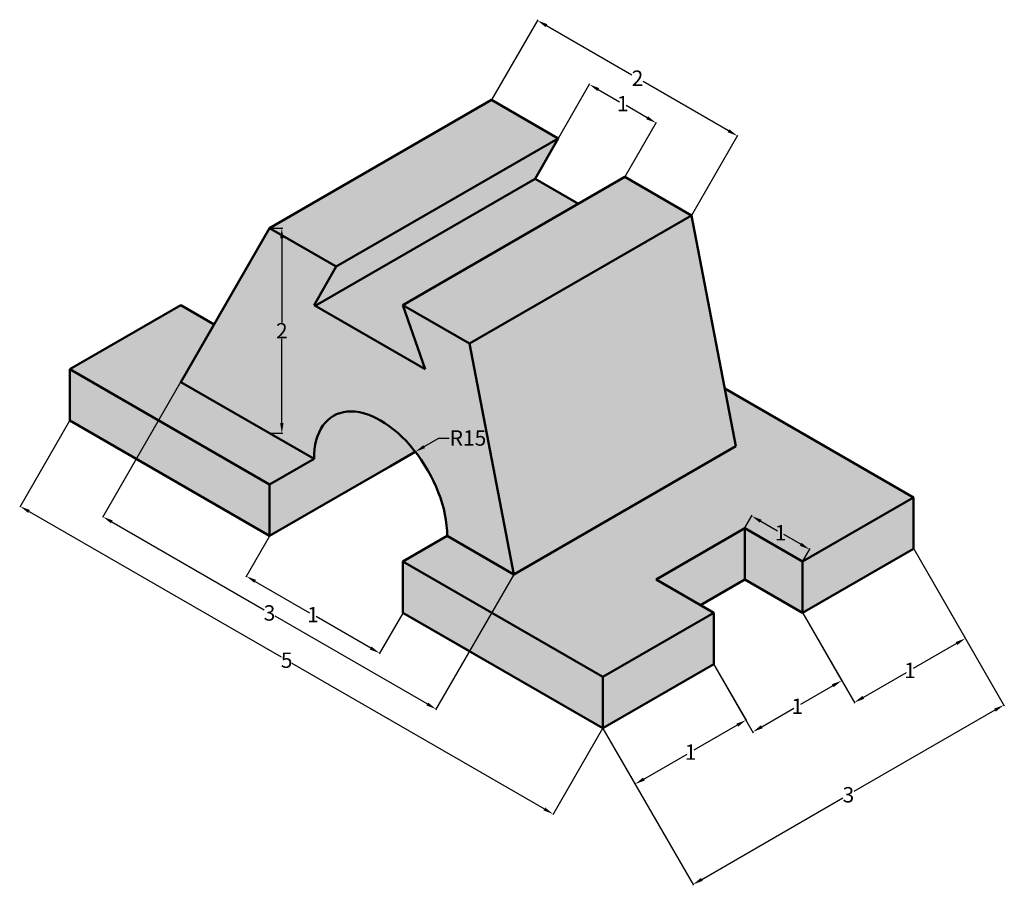
# Model space of a CAD drawing. Units: inches. Extents: x 162 to 354, y 120 to 289.
import ezdxf
from ezdxf import colors
from ezdxf.entities.mleader import LeaderData, LeaderLine
from ezdxf.math import Vec2, Vec3

# ---------------------------------------------------------------- set-up
doc = ezdxf.new("R2010")
doc.units = ezdxf.units.IN
doc.header["$MEASUREMENT"] = 0
for name, color, linetype, lineweight in [('M-DIMS', 2, 'Continuous', 25), ('M-HATC', 252, 'Continuous', 18), ('M-OUTL', 7, 'Continuous', 50), ('M-TEXT', 7, 'Continuous', 25)]:
    doc.layers.add(name, color=color, linetype=linetype, lineweight=lineweight)
doc.styles.get("Standard").update_dxf_attribs({"font": 'arial.ttf'})
doc.dimstyles.get("Standard").update_dxf_attribs({"dimtxt": 3, "dimasz": 2, "dimexe": 0.18, "dimexo": 0.0625, "dimgap": 0.09, "dimtad": 0, "dimtih": 1, "dimtoh": 1, "dimdec": 0, "dimzin": 0, "dimdsep": 46, "dimtxsty": 'Standard', "dimcen": 0.09, "dimadec": 0, "dimazin": 0, "dimtfac": 1, "dimtdec": 0, "dimtofl": 0, "dimtmove": 0, "dimatfit": 3, "dimfxl": 1, "dimtolj": 1, "dimtzin": 0, "dimarcsym": 0})

# ---------------------------------------------------------------- blocks, each defined once
blk = doc.blocks.new('*D23')
at = {"layer": 'Defpoints', "color": 0, "transparency": 16777216}
for p in [(172.0397916164236, 210.9806443557733), (275.9628400705561, 150.9806443557734), (266.299650434846, 134.2435089435503)]:
    blk.add_point(p, dxfattribs=at)
at = {"layer": 'M-DIMS', "color": 0, "lineweight": -2, "transparency": 16777216}
for p, q in [((172.0085416164236, 210.9265177680369), (162.2866019807134, 194.0876243708691)), ((164.1086527882822, 193.2435089435503), (213.2535832337005, 164.8696701215826)), ((264.5675996272771, 135.2435089435503), (215.4226691818588, 163.617347765518)), ((275.9315900705561, 150.9265177680369), (266.2096504348459, 134.0876243708691))]:
    blk.add_line(p, q, dxfattribs=at)
at = {"layer": 'M-DIMS', "color": 0, "transparency": 16777216}
for points in [[(164.2753194549489, 193.5321840781451), (163.9419861216156, 192.9548338089555), (162.3766019807134, 194.2435089435503)], [(264.7342662939437, 135.5321840781451), (264.4009329606104, 134.9548338089554), (266.299650434846, 134.2435089435503)]]:
    blk.add_solid(points, dxfattribs=at)
at = {"layer": 'M-DIMS', "color": 0, "transparency": 16777216, "insert": (214.3381262077797, 164.2435089435503), "char_height": 3, "attachment_point": 5}
blk.add_mtext('\\A1;5', dxfattribs=at)
blk = doc.blocks.new('*D24')
at = {"layer": 'Defpoints', "color": 0, "transparency": 16777216}
for p in [(297.6134751651672, 163.4806443557734), (275.9628400705562, 150.9806443557733), (282.2602066725913, 140.0732854471611)]:
    blk.add_point(p, dxfattribs=at)
at = {"layer": 'M-DIMS', "color": 0, "lineweight": -2, "transparency": 16777216}
for p, q in [((297.6447251651673, 163.4265177680368), (304.0008417672023, 152.4174008744799)), ((275.9940900705562, 150.9265177680368), (282.3502066725913, 139.9174008744799)), ((302.1787909596335, 151.5732854471611), (293.7280480943853, 146.6942467790578)), ((283.9922574801601, 141.0732854471611), (292.4430003454085, 145.9523241152645))]:
    blk.add_line(p, q, dxfattribs=at)
at = {"layer": 'M-DIMS', "color": 0, "transparency": 16777216}
for points in [[(302.0121242929668, 151.8619605817559), (302.3454576263001, 151.2846103125663), (303.9108417672024, 152.5732854471611)], [(283.8255908134935, 141.3619605817559), (284.1589241468268, 140.7846103125663), (282.2602066725913, 140.0732854471611)]]:
    blk.add_solid(points, dxfattribs=at)
at = {"layer": 'M-DIMS', "color": 0, "transparency": 16777216, "insert": (293.0855242198969, 146.3232854471611), "char_height": 3, "attachment_point": 5}
blk.add_mtext('\\A1;1', dxfattribs=at)
blk = doc.blocks.new('*D25')
at = {"layer": 'Defpoints', "color": 0, "transparency": 16777216}
for p in [(336.5846183354669, 185.9806443557734), (314.9339832408559, 173.4806443557733), (325.0300341251803, 155.9937712683226)]:
    blk.add_point(p, dxfattribs=at)
at = {"layer": 'M-DIMS', "color": 0, "lineweight": -2, "transparency": 16777216}
for p, q in [((336.6158683354669, 185.9265177680368), (346.7706692197914, 168.3378866956414)), ((314.9652332408559, 173.4265177680368), (325.1200341251804, 155.8378866956414)), ((344.9486184122225, 167.4937712683227), (336.4978755469742, 162.6147326002192)), ((326.7620849327493, 156.9937712683226), (335.2128277979974, 161.872809936426))]:
    blk.add_line(p, q, dxfattribs=at)
at = {"layer": 'M-DIMS', "color": 0, "transparency": 16777216}
for points in [[(344.7819517455559, 167.7824464029175), (345.1152850788892, 167.2050961337278), (346.6806692197914, 168.4937712683226)], [(326.5954182660826, 157.2824464029174), (326.9287515994159, 156.7050961337278), (325.0300341251803, 155.9937712683226)]]:
    blk.add_solid(points, dxfattribs=at)
at = {"layer": 'M-DIMS', "color": 0, "transparency": 16777216, "insert": (335.8553516724858, 162.2437712683226), "char_height": 3, "attachment_point": 5}
blk.add_mtext('\\A1;1', dxfattribs=at)
blk = doc.blocks.new('*D26')
at = {"layer": 'Defpoints', "color": 0, "transparency": 16777216}
for p in [(314.933983240856, 173.4806443557734), (297.6134751651672, 163.4806443557734), (322.562421822814, 160.2678011494034)]:
    blk.add_point(p, dxfattribs=at)
at = {"layer": 'M-DIMS', "color": 0, "lineweight": -2, "transparency": 16777216}
for p, q in [((314.965233240856, 173.4265177680368), (322.6524218228141, 160.1119165767221)), ((297.6447251651673, 163.4265177680369), (305.3319137471253, 150.1119165767222)), ((320.8303710152451, 159.2678011494033), (314.5446916594581, 155.6387624813)), ((306.9739645546942, 151.2678011494034), (313.2596439104813, 154.8968398175067))]:
    blk.add_line(p, q, dxfattribs=at)
at = {"layer": 'M-DIMS', "color": 0, "transparency": 16777216}
for points in [[(320.6637043485784, 159.5564762839982), (320.9970376819118, 158.9791260148085), (322.562421822814, 160.2678011494034)], [(306.8072978880275, 151.5564762839982), (307.1406312213609, 150.9791260148086), (305.2419137471253, 150.2678011494034)]]:
    blk.add_solid(points, dxfattribs=at)
at = {"layer": 'M-DIMS', "color": 0, "transparency": 16777216, "insert": (313.9021677849697, 155.2678011494033), "char_height": 3, "attachment_point": 5}
blk.add_mtext('\\A1;1', dxfattribs=at)
blk = doc.blocks.new('*D27')
at = {"layer": 'Defpoints', "color": 0, "transparency": 16777216}
for p in [(336.584618335467, 185.9806443557733), (354.1777602048822, 155.5084287731787), (275.9628400705562, 150.9806443557734)]:
    blk.add_point(p, dxfattribs=at)
at = {"layer": 'M-DIMS', "color": 0, "lineweight": -2, "transparency": 16777216}
for p, q in [((336.6158683354669, 185.9265177680368), (354.2677602048822, 155.3525442004975)), ((352.4457093973134, 154.5084287731787), (324.939135738184, 138.6275010665962)), ((275.9940900705562, 150.9265177680369), (293.6459819399715, 120.3525442004976)), ((295.2880327475404, 121.5084287731788), (322.7946064066697, 137.3893564797614))]:
    blk.add_line(p, q, dxfattribs=at)
at = {"layer": 'M-DIMS', "color": 0, "transparency": 16777216}
for points in [[(352.2790427306467, 154.7971039077736), (352.6123760639801, 154.219753638584), (354.1777602048822, 155.5084287731787)], [(295.1213660808737, 121.7971039077736), (295.4546994142071, 121.2197536385839), (293.5559819399715, 120.5084287731787)]]:
    blk.add_solid(points, dxfattribs=at)
at = {"layer": 'M-DIMS', "color": 0, "transparency": 16777216, "insert": (323.8668710724269, 138.0084287731787), "char_height": 3, "attachment_point": 5}
blk.add_mtext('\\A1;3', dxfattribs=at)
blk = doc.blocks.new('*D28')
at = {"layer": 'Defpoints', "color": 0, "transparency": 16777216}
for p in [(286.367162029734, 269.0014586073739), (267.3025860327118, 265.9806443557734), (280.2929670894784, 258.4806443557734)]:
    blk.add_point(p, dxfattribs=at)
at = {"layer": 'M-DIMS', "color": 0, "lineweight": -2, "transparency": 16777216}
for p, q in [((267.3338360327118, 266.03477094351), (273.4667809729675, 276.6573431800551)), ((275.1088317805363, 275.5014586073739), (279.2294476268623, 273.1224199392705)), ((284.6351112221652, 270.0014586073739), (280.5144953758391, 272.3804972754773)), ((280.3242170894784, 258.53477094351), (286.457162029734, 269.1573431800551))]:
    blk.add_line(p, q, dxfattribs=at)
at = {"layer": 'M-DIMS', "color": 0, "transparency": 16777216}
for points in [[(275.275498447203, 275.7901337419687), (274.9421651138696, 275.2127834727791), (273.3767809729674, 276.5014586073739)], [(284.8017778888318, 270.2901337419687), (284.4684445554985, 269.7127834727791), (286.367162029734, 269.0014586073739)]]:
    blk.add_solid(points, dxfattribs=at)
at = {"layer": 'M-DIMS', "color": 0, "transparency": 16777216, "insert": (279.8719715013507, 272.7514586073739), "char_height": 3, "attachment_point": 5}
blk.add_mtext('\\A1;1', dxfattribs=at)
blk = doc.blocks.new('*D29')
at = {"layer": 'Defpoints', "color": 0, "transparency": 16777216}
for p in [(254.3122049759452, 273.4806443557734), (302.2288190770284, 266.4746545055207), (293.283348146245, 250.9806443557734)]:
    blk.add_point(p, dxfattribs=at)
at = {"layer": 'M-DIMS', "color": 0, "lineweight": -2, "transparency": 16777216}
for p, q in [((254.3434549759452, 273.5347709435099), (263.3476759067286, 289.1305390782019)), ((264.9897267142975, 287.9746545055207), (281.6597277101595, 278.3502249431685)), ((300.4967682694595, 267.4746545055207), (283.8267672735975, 277.099084067873)), ((293.314598146245, 251.0347709435099), (302.3188190770284, 266.630539078202))]:
    blk.add_line(p, q, dxfattribs=at)
at = {"layer": 'M-DIMS', "color": 0, "transparency": 16777216}
for points in [[(265.1563933809641, 288.2633296401156), (264.8230600476308, 287.685979370926), (263.2576759067286, 288.9746545055207)], [(300.6634349361262, 267.7633296401156), (300.3301016027929, 267.185979370926), (302.2288190770284, 266.4746545055207)]]:
    blk.add_solid(points, dxfattribs=at)
at = {"layer": 'M-DIMS', "color": 0, "transparency": 16777216, "insert": (282.7432474918785, 277.7246545055207), "char_height": 3, "attachment_point": 5}
blk.add_mtext('\\A1;2', dxfattribs=at)
blk = doc.blocks.new('*D30')
at = {"layer": 'Defpoints', "color": 0, "transparency": 16777216}
for p in [(211.0109347867234, 248.4806443557735), (211.0109347867234, 208.4806443557735), (213.3940942620055, 208.4806443557735)]:
    blk.add_point(p, dxfattribs=at)
at = {"layer": 'M-DIMS', "color": 0, "lineweight": -2, "transparency": 16777216}
for p, q in [((211.0734347867234, 248.4806443557735), (213.5740942620055, 248.4806443557735)), ((213.3940942620055, 246.4806443557735), (213.3940942620055, 230.0767835099345)), ((213.3940942620055, 210.4806443557735), (213.3940942620055, 226.8845052016125)), ((211.0734347867234, 208.4806443557735), (213.5740942620055, 208.4806443557735))]:
    blk.add_line(p, q, dxfattribs=at)
at = {"layer": 'M-DIMS', "color": 0, "transparency": 16777216}
for points in [[(213.0607609286721, 246.4806443557735), (213.7274275953388, 246.4806443557735), (213.3940942620055, 248.4806443557735)], [(213.0607609286721, 210.4806443557735), (213.7274275953388, 210.4806443557735), (213.3940942620055, 208.4806443557735)]]:
    blk.add_solid(points, dxfattribs=at)
at = {"layer": 'M-DIMS', "color": 0, "transparency": 16777216, "insert": (213.3940942620055, 228.4806443557734), "char_height": 3, "attachment_point": 5}
blk.add_mtext('\\A1;2', dxfattribs=at)
blk = doc.blocks.new('*D31')
at = {"layer": 'Defpoints', "color": 0, "transparency": 16777216}
for p in [(211.0109347867233, 188.4806443557734), (236.9916969002565, 173.4806443557735), (232.4520416852814, 165.6177308745916)]:
    blk.add_point(p, dxfattribs=at)
at = {"layer": 'M-DIMS', "color": 0, "lineweight": -2, "transparency": 16777216}
for p, q in [((210.9796847867233, 188.4265177680368), (206.3812795717482, 180.4618463019102)), ((208.2033303793171, 179.6177308745915), (218.8191367540264, 173.4886922064881)), ((236.9604469002565, 173.4265177680369), (232.3620416852814, 165.4618463019104)), ((230.7199908777125, 166.6177308745916), (220.1041845030033, 172.7467695426949))]:
    blk.add_line(p, q, dxfattribs=at)
at = {"layer": 'M-DIMS', "color": 0, "transparency": 16777216}
for points in [[(208.3699970459838, 179.9064060091863), (208.0366637126505, 179.3290557399967), (206.4712795717482, 180.6177308745914)], [(230.8866575443792, 166.9064060091864), (230.5533242110459, 166.3290557399968), (232.4520416852814, 165.6177308745916)]]:
    blk.add_solid(points, dxfattribs=at)
at = {"layer": 'M-DIMS', "color": 0, "transparency": 16777216, "insert": (219.4616606285148, 173.1177308745915), "char_height": 3, "attachment_point": 5}
blk.add_mtext('\\A1;1', dxfattribs=at)
blk = doc.blocks.new('*D32')
at = {"layer": 'Defpoints', "color": 0, "transparency": 16777216}
for p in [(193.6904267110344, 218.4806443557734), (258.6423319948675, 180.9806443557734), (243.4751159444774, 154.7102555471235)]:
    blk.add_point(p, dxfattribs=at)
at = {"layer": 'M-DIMS', "color": 0, "lineweight": -2, "transparency": 16777216}
for p, q in [((193.6591767110344, 218.4265177680368), (178.4332106606444, 192.0543709744423)), ((180.2552614682132, 191.2102555471235), (209.9268986368037, 174.079327840541)), ((258.6110819948675, 180.9265177680368), (243.3851159444774, 154.5543709744423)), ((241.7430651369085, 155.7102555471235), (212.071427968318, 172.8411832537061))]:
    blk.add_line(p, q, dxfattribs=at)
at = {"layer": 'M-DIMS', "color": 0, "transparency": 16777216}
for points in [[(180.4219281348799, 191.4989306817183), (180.0885948015466, 190.9215804125287), (178.5232106606444, 192.2102555471235)], [(241.9097318035752, 155.9989306817183), (241.5763984702418, 155.4215804125287), (243.4751159444774, 154.7102555471235)]]:
    blk.add_solid(points, dxfattribs=at)
at = {"layer": 'M-DIMS', "color": 0, "transparency": 16777216, "insert": (210.9991633025609, 173.4602555471235), "char_height": 3, "attachment_point": 5}
blk.add_mtext('\\A1;3', dxfattribs=at)
blk = doc.blocks.new('*D33')
at = {"layer": 'Defpoints', "color": 0, "transparency": 16777216}
for p in [(303.6756529916583, 189.9806443557734), (316.2979778399645, 185.8431523026789), (314.9339832408559, 183.4806443557734)]:
    blk.add_point(p, dxfattribs=at)
at = {"layer": 'M-DIMS', "color": 0, "lineweight": -2, "transparency": 16777216}
for p, q in [((303.7069029916583, 190.0347709435099), (305.1296475907669, 192.4990368753601)), ((306.7716983983357, 191.3431523026789), (310.0262888408773, 189.4641136345755)), ((314.5659270323956, 186.8431523026789), (311.3113365898541, 188.7221909707822)), ((314.9652332408559, 183.5347709435099), (316.3879778399645, 185.9990368753601))]:
    blk.add_line(p, q, dxfattribs=at)
at = {"layer": 'M-DIMS', "color": 0, "transparency": 16777216}
for points in [[(306.9383650650024, 191.6318274372737), (306.6050317316691, 191.0544771680841), (305.0396475907669, 192.3431523026789)], [(314.7325936990622, 187.1318274372737), (314.3992603657289, 186.5544771680841), (316.2979778399645, 185.8431523026789)]]:
    blk.add_solid(points, dxfattribs=at)
at = {"layer": 'M-DIMS', "color": 0, "transparency": 16777216, "insert": (310.6688127153657, 189.0931523026789), "char_height": 3, "attachment_point": 5}
blk.add_mtext('\\A1;1', dxfattribs=at)

msp = doc.modelspace()

# ---------------------------------------------------------------- hatches: boundary and pattern name
at = {"layer": 'M-HATC'}
h = msp.add_hatch(color=256, dxfattribs=at)
h.dxf.hatch_style = 1
edge = h.paths.add_edge_path()
edge.add_line((219.6711888245677, 233.4806443557734), (224.0013158434899, 240.9806443557734))
edge.add_line((224.0013158434899, 240.9806443557734), (211.0109347867233, 248.4806443557734))
edge.add_line((211.0109347867233, 248.4806443557734), (193.6904267110345, 218.4806443557735))
edge.add_line((193.6904267110345, 218.4806443557735), (219.6711888245677, 203.4806443557734))
edge.add_ellipse((232.6615698813343, 195.9806443557734), major_axis=(9.185586535436935, -15.90990257669732), ratio=0.5773502691896266, start_angle=509.9999999999998, end_angle=570.0000000000001, ccw=False)
edge.add_ellipse((232.6615698813343, 195.9806443557734), major_axis=(9.185586535436935, -15.90990257669732), ratio=0.5773502691896266, start_angle=472.7864979995972, end_angle=509.9999999999998, ccw=False)
edge.add_ellipse((232.6615698813343, 195.9806443557734), major_axis=(9.185586535436935, -15.90990257669732), ratio=0.5773502691896266, start_angle=389.99999999999994, end_angle=472.7864979995972, ccw=False)
edge.add_line((245.6519509381009, 188.4806443557734), (258.6423319948675, 180.9806443557734))
edge.add_line((258.6423319948675, 180.9806443557734), (249.982077957023, 225.9806443557734))
edge.add_line((249.982077957023, 225.9806443557734), (236.9916969002565, 233.4806443557734))
edge.add_line((236.9916969002565, 233.4806443557734), (241.3218239191786, 220.9806443557734))
edge.add_line((241.3218239191786, 220.9806443557734), (219.6711888245677, 233.4806443557734))
h.paths.add_polyline_path([(200.1856172394179, 229.7306443557735), (193.6904267110346, 233.4806443557734), (172.0397916164236, 220.9806443557734), (211.0109347867233, 198.4806443557734), (219.6711888245677, 203.4806443557734), (193.6904267110345, 218.4806443557735)])
h.paths.add_polyline_path([(236.9916969002565, 183.4806443557734), (236.9916969002565, 173.4806443557734), (249.9820779570231, 165.9806443557734), (275.9628400705562, 150.9806443557734), (275.9628400705562, 160.9806443557734)])
h.paths.add_polyline_path([(211.0109347867233, 198.4806443557734), (172.0397916164236, 220.9806443557734), (172.0397916164236, 210.9806443557734), (211.0109347867233, 188.4806443557734)])
h.paths.add_polyline_path([(293.283348146245, 250.9806443557734), (280.2929670894784, 258.4806443557734), (236.9916969002565, 233.4806443557734), (249.982077957023, 225.9806443557734)])
h.paths.add_polyline_path([(267.3025860327118, 265.9806443557734), (254.3122049759452, 273.4806443557734), (211.0109347867233, 248.4806443557734), (224.0013158434899, 240.9806443557734)])
h.paths.add_polyline_path([(286.3551449159695, 179.9806443557734), (303.6756529916583, 189.9806443557734), (314.9339832408559, 183.4806443557734), (336.5846183354669, 195.9806443557734), (299.7785386746283, 217.2306443557733), (301.9436021840894, 205.9806443557735), (258.6423319948675, 180.9806443557734), (245.6519509381009, 188.4806443557734), (236.9916969002565, 183.4806443557734), (275.9628400705562, 160.9806443557734), (297.6134751651672, 173.4806443557734)])
h.paths.add_polyline_path([(314.9339832408559, 183.4806443557734), (303.6756529916583, 189.9806443557734), (303.6756529916583, 179.9806443557734), (314.9339832408559, 173.4806443557734)], flags=17)
h = msp.add_hatch(color=256, dxfattribs=at)
h.dxf.hatch_style = 1
h.paths.add_polyline_path([(271.2276956603566, 253.2468074558929), (262.769950318151, 258.1298890059527), (219.8736975202064, 233.3637259058331), (241.3218239191786, 220.9806443557734), (236.9916969002565, 233.4806443557734)])
h.paths.add_polyline_path([(262.769950318151, 258.1298890059527), (267.3025860327118, 265.9806443557734), (224.0013158434899, 240.9806443557734), (219.8875971121148, 233.8554745049839), (219.8736975202064, 233.3637259058332)])
edge = h.paths.add_edge_path()
edge.add_ellipse((232.6615698813343, 195.9806443557734), major_axis=(9.185586535436935, -15.90990257669732), ratio=0.5773502691896266, start_angle=509.9999999999998, end_angle=210.0000000000001)
edge.add_line((219.6711888245677, 203.4806443557734), (232.6615698813343, 210.9806443557734))
edge = h.paths.add_edge_path()
edge.add_line((234.5601018929612, 202.0767623237514), (239.4232919075518, 204.8845263877955))
edge.add_ellipse((232.6615698813343, 195.9806443557734), major_axis=(9.185586535436935, -15.90990257669732), ratio=0.5773502691896266, start_angle=472.7864979995971, end_angle=509.9999999999998)
edge.add_line((232.6615698813343, 210.9806443557734), (219.6711888245677, 203.4806443557734))
edge.add_line((219.6711888245677, 203.4806443557734), (211.0109347867233, 198.4806443557734))
edge.add_line((211.0109347867233, 198.4806443557734), (211.0109347867233, 188.4806443557734))
edge.add_line((211.0109347867233, 188.4806443557734), (221.5697208361946, 194.5767623237513))
edge.add_line((221.5697208361946, 194.5767623237513), (234.5601018929612, 202.0767623237514))
h.paths.add_polyline_path([(297.6134751651672, 173.4806443557734), (275.9628400705562, 160.9806443557734), (275.9628400705562, 150.9806443557734), (297.6134751651672, 163.4806443557734)])
h.paths.add_polyline_path([(301.9436021840894, 205.9806443557735), (293.283348146245, 250.9806443557734), (249.982077957023, 225.9806443557734), (258.6423319948675, 180.9806443557734)])
h.paths.add_polyline_path([(303.6756529916583, 179.9806443557734), (303.6756529916583, 189.9806443557734), (286.3551449159695, 179.9806443557734), (295.0153989538139, 174.9806443557734)])
h.paths.add_polyline_path([(336.5846183354669, 185.9806443557734), (336.5846183354669, 195.9806443557734), (314.9339832408559, 183.4806443557734), (314.9339832408559, 173.4806443557734)])

# ---------------------------------------------------------------- linework, layer by layer
at = {"layer": 'M-OUTL'}
for p, q in [((211.0109347867233, 248.4806443557734), (254.3122049759452, 273.4806443557734)), ((254.3122049759452, 273.4806443557734), (267.3025860327118, 265.9806443557734)), ((267.3025860327118, 265.9806443557734), (224.0013158434899, 240.9806443557734)), ((262.769950318151, 258.1298890059527), (267.3025860327118, 265.9806443557734)), ((219.8736975202064, 233.3637259058332), (262.769950318151, 258.1298890059527)), ((236.9916969002565, 233.4806443557734), (280.2929670894784, 258.4806443557734)), ((262.769950318151, 258.1298890059527), (271.2276956603566, 253.2468074558929)), ((280.2929670894784, 258.4806443557734), (293.283348146245, 250.9806443557734)), ((249.982077957023, 225.9806443557734), (293.283348146245, 250.9806443557734)), ((293.283348146245, 250.9806443557734), (301.9436021840894, 205.9806443557735)), ((211.0109347867233, 248.4806443557734), (193.6904267110345, 218.4806443557735)), ((224.0013158434899, 240.9806443557734), (211.0109347867233, 248.4806443557734)), ((284.2180767171232, 245.7468074558929), (284.4205854127619, 245.6298890059527)), ((224.0013158434899, 240.9806443557734), (219.6711888245677, 233.4806443557734)), ((172.0397916164236, 220.9806443557734), (193.6904267110346, 233.4806443557734)), ((193.6904267110346, 233.4806443557734), (200.1856172394178, 229.7306443557735)), ((219.6711888245677, 233.4806443557734), (241.3218239191786, 220.9806443557734)), ((219.8875971121148, 233.855474504984), (219.8736975202064, 233.3637259058331)), ((236.9916969002565, 233.4806443557734), (241.3218239191786, 220.9806443557734)), ((236.9916969002565, 233.4806443557734), (249.982077957023, 225.9806443557734)), ((249.982077957023, 225.9806443557734), (258.6423319948675, 180.9806443557734)), ((172.0397916164236, 210.9806443557734), (172.0397916164236, 220.9806443557734)), ((172.0397916164236, 220.9806443557734), (211.0109347867233, 198.4806443557735)), ((219.6711888245677, 203.4806443557734), (193.6904267110345, 218.4806443557734)), ((336.5846183354669, 195.9806443557734), (299.7785386746283, 217.2306443557733)), ((211.0109347867233, 188.4806443557734), (172.0397916164236, 210.9806443557734)), ((219.6711888245677, 203.4806443557734), (211.0109347867233, 208.4806443557734)), ((258.6423319948675, 180.9806443557734), (301.9436021840894, 205.9806443557735)), ((234.5601018929612, 202.0767623237514), (239.4232919075518, 204.8845263877955)), ((219.6711888245677, 203.4806443557734), (211.0109347867233, 198.4806443557734)), ((221.5697208361946, 194.5767623237513), (234.5601018929612, 202.0767623237514)), ((211.0109347867233, 188.4806443557734), (211.0109347867233, 198.4806443557734)), ((211.0109347867233, 188.4806443557734), (198.0205537299567, 195.9806443557734)), ((336.5846183354669, 195.9806443557734), (314.9339832408559, 183.4806443557734)), ((336.5846183354669, 185.9806443557734), (336.5846183354669, 195.9806443557734)), ((211.0109347867233, 188.4806443557734), (221.5697208361946, 194.5767623237513)), ((236.9916969002565, 183.4806443557734), (245.6519509381009, 188.4806443557734)), ((245.6519509381009, 188.4806443557734), (258.6423319948675, 180.9806443557734)), ((286.3551449159695, 179.9806443557734), (303.6756529916583, 189.9806443557734)), ((303.6756529916583, 189.9806443557734), (314.9339832408559, 183.4806443557734)), ((303.6756529916583, 179.9806443557734), (303.6756529916583, 189.9806443557734)), ((314.9339832408559, 173.4806443557734), (336.5846183354669, 185.9806443557734)), ((236.9916969002565, 173.4806443557734), (236.9916969002565, 183.4806443557734)), ((236.9916969002565, 183.4806443557734), (275.9628400705562, 160.9806443557734)), ((314.9339832408559, 183.4806443557734), (314.9339832408559, 173.4806443557734)), ((297.6134751651672, 173.4806443557734), (286.3551449159695, 179.9806443557734)), ((303.6756529916583, 179.9806443557734), (295.0153989538139, 174.9806443557734)), ((314.9339832408559, 173.4806443557734), (303.6756529916583, 179.9806443557734)), ((275.9628400705562, 150.9806443557734), (236.9916969002565, 173.4806443557735)), ((236.9916969002565, 173.4806443557734), (249.9820779570231, 165.9806443557734)), ((275.9628400705562, 160.9806443557734), (297.6134751651672, 173.4806443557734)), ((297.6134751651672, 163.4806443557734), (297.6134751651672, 173.4806443557734)), ((275.9628400705562, 150.9806443557734), (297.6134751651672, 163.4806443557734)), ((275.9628400705562, 160.9806443557734), (275.9628400705562, 150.9806443557734))]:
    msp.add_line(p, q, dxfattribs=at)
msp.add_ellipse((232.6615698813343, 195.9806443557734), major_axis=(9.18558653543693, -15.90990257669731), ratio=0.5773502691896267, start_param=7.068583470577032, end_param=10.21017612416683, dxfattribs=at)

# ---------------------------------------------------------------- dimensions: what is measured, and where the dimension line sits
at = {"layer": 'M-DIMS'}
for base, p1, p2, angle, picture, middle in [((302.2288190770284, 266.4746545055207), (254.3122049759452, 273.4806443557734), (293.283348146245, 250.9806443557734), 330.0000000000001, '*D29', (282.7432474918785, 277.7246545055207)), ((286.367162029734, 269.0014586073739), (267.3025860327118, 265.9806443557734), (280.2929670894784, 258.4806443557734), 330, '*D28', (279.8719715013507, 272.7514586073739)), ((213.3940942620055, 208.4806443557735), (211.0109347867233, 248.4806443557734), (211.0109347867233, 208.4806443557734), 270, '*D30', (213.3940942620055, 228.4806443557734)), ((243.4751159444774, 154.7102555471235), (193.6904267110345, 218.4806443557734), (258.6423319948675, 180.9806443557734), 330.0000000000001, '*D32', (210.9991633025609, 173.4602555471235)), ((266.299650434846, 134.2435089435503), (172.0397916164236, 210.9806443557734), (275.9628400705562, 150.9806443557734), 330, '*D23', (214.3381262077797, 164.2435089435503)), ((316.2979778399645, 185.8431523026789), (303.6756529916583, 189.9806443557734), (314.9339832408559, 183.4806443557734), 329.9999999999998, '*D33', (310.6688127153657, 189.0931523026789)), ((232.4520416852814, 165.6177308745916), (211.0109347867233, 188.4806443557734), (236.9916969002565, 173.4806443557735), 330.0000000000002, '*D31', (219.4616606285148, 173.1177308745915)), ((354.1777602048822, 155.5084287731787), (275.9628400705562, 150.9806443557734), (336.584618335467, 185.9806443557734), 29.99999999999999, '*D27', (323.8668710724269, 138.0084287731787)), ((325.0300341251803, 155.9937712683226), (336.584618335467, 185.9806443557734), (314.9339832408559, 173.4806443557734), 210, '*D25', (335.8553516724858, 162.2437712683226)), ((322.562421822814, 160.2678011494034), (297.6134751651672, 163.4806443557734), (314.9339832408559, 173.4806443557734), 30.00000000000005, '*D26', (313.9021677849697, 155.2678011494033)), ((282.2602066725913, 140.0732854471611), (297.6134751651672, 163.4806443557734), (275.9628400705562, 150.9806443557734), 210, '*D24', (293.0855242198969, 146.3232854471611))]:
    dim = msp.add_linear_dim(base=base, p1=p1, p2=p2, angle=angle, dimstyle='Standard', override={"dimlfac": 0.0393700787401575, "dimrnd": 0}, dxfattribs=at)
    dim.commit()
    dim.dimension.update_dxf_attribs({"geometry": picture, "text_midpoint": middle})

# ---------------------------------------------------------------- leaders
at = {"layer": 'M-TEXT'}
ml = msp.add_multileader_mtext('Standard', dxfattribs=at)
ml.set_content('R15', color=256)
ml.set_leader_properties()
ml.build(insert=Vec2(0, 0))
ml.multileader.update_dxf_attribs({"dogleg_length": 2, "arrow_head_size": 2})
ctx = ml.context
ctx.base_point, ctx.char_height, ctx.arrow_head_size, ctx.landing_gap_size, ctx.plane_origin = Vec3(246.0303332920448, 207.5444029713004), 3, 2, 0.09, Vec3(239.4232919075518, 204.8845263877955)
notes = []
notes.append((ctx, [(0, (1, 1, 0), (244.0303332920448, 207.5444029713004), (1, 0), 2, [(0, [(239.4232919075518, 204.8845263877955)], 0, [])])]))
ctx.mtext.insert, ctx.mtext.flow_direction = Vec3(246.1203332920448, 209.0699827803044), 5
for ctx, leaders in notes:
    for number, flags, end, landing, length, lines in leaders:
        leader = LeaderData()
        leader.index, (leader.has_last_leader_line, leader.has_dogleg_vector, leader.attachment_direction) = number, flags
        leader.last_leader_point, leader.dogleg_vector, leader.dogleg_length = Vec3(end), Vec3(landing), length
        for number, points, colour, breaks in lines:
            line = LeaderLine()
            line.index, line.vertices, line.color, line.breaks = number, Vec3.list(points), colors.encode_raw_color(colour), breaks
            leader.lines.append(line)
        ctx.leaders.append(leader)

doc.saveas('drawing.dxf')
